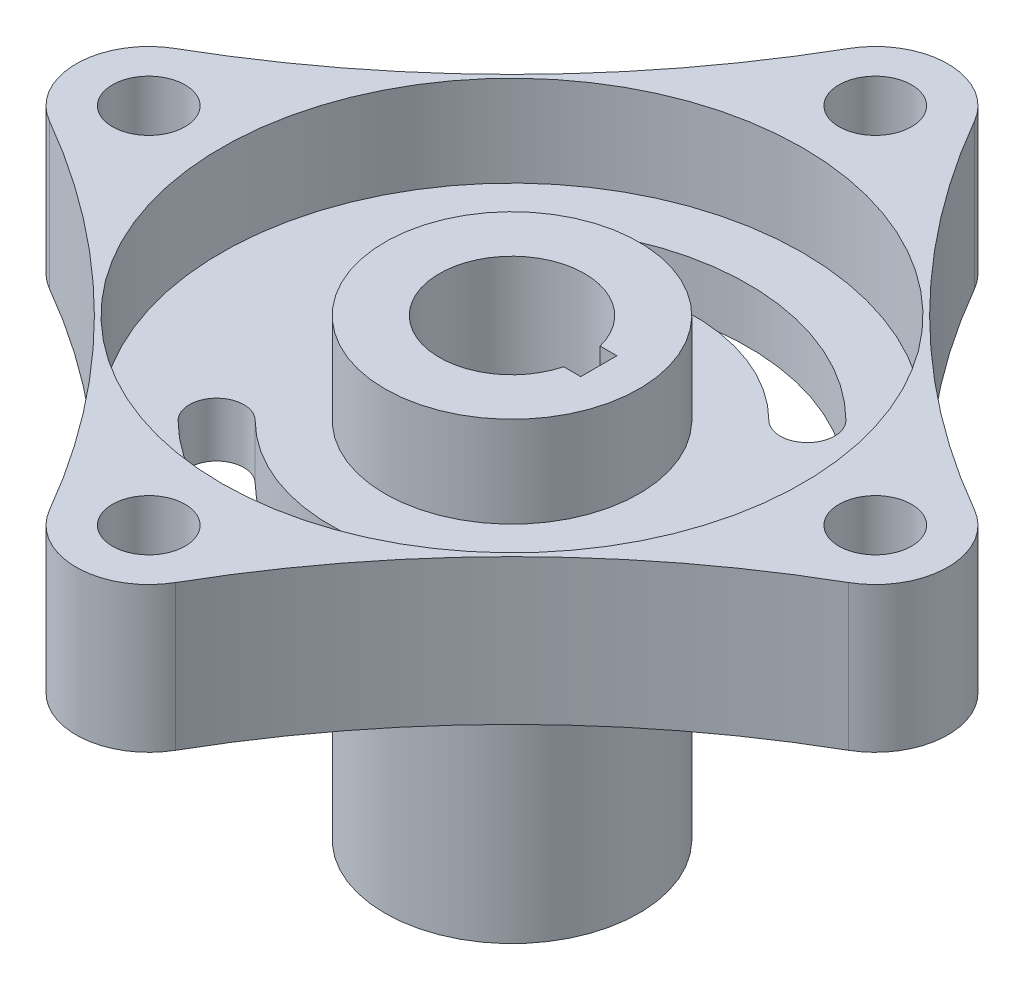
ISO-10303-21;
HEADER;
FILE_DESCRIPTION(('STEP AP214'),'2;1');
FILE_NAME('part.step','',(''),(''),'','','');
FILE_SCHEMA(('AUTOMOTIVE_DESIGN { 1 0 10303 214 1 1 1 1 }'));
ENDSEC;
DATA;
#1=APPLICATION_CONTEXT('core data for automotive mechanical design processes');
#2=APPLICATION_PROTOCOL_DEFINITION('international standard','automotive_design',2000,#1);
#3=PRODUCT_CONTEXT('',#1,'mechanical');
#4=PRODUCT('Part','Part','',(#3));
#5=PRODUCT_RELATED_PRODUCT_CATEGORY('part','',(#4));
#6=PRODUCT_DEFINITION_FORMATION('','',#4);
#7=PRODUCT_DEFINITION_CONTEXT('part definition',#1,'design');
#8=PRODUCT_DEFINITION('design','',#6,#7);
#9=PRODUCT_DEFINITION_SHAPE('','',#8);
#10=(LENGTH_UNIT() NAMED_UNIT(*) SI_UNIT(.MILLI.,.METRE.));
#11=(NAMED_UNIT(*) PLANE_ANGLE_UNIT() SI_UNIT($,.RADIAN.));
#12=(NAMED_UNIT(*) SI_UNIT($,.STERADIAN.) SOLID_ANGLE_UNIT());
#13=UNCERTAINTY_MEASURE_WITH_UNIT(LENGTH_MEASURE(1.E-05),#10,'distance_accuracy_value','');
#14=(GEOMETRIC_REPRESENTATION_CONTEXT(3) GLOBAL_UNCERTAINTY_ASSIGNED_CONTEXT((#13)) GLOBAL_UNIT_ASSIGNED_CONTEXT((#10,
#11,#12)) REPRESENTATION_CONTEXT('',''));
#15=CARTESIAN_POINT('',(0.,0.,0.));
#16=DIRECTION('',(0.,0.,1.));
#17=DIRECTION('',(1.,0.,0.));
#18=AXIS2_PLACEMENT_3D('',#15,#16,#17);
#19=CARTESIAN_POINT('',(66.8510515453765,0.,-46.8510515453766));
#20=DIRECTION('',(0.,1.,0.));
#21=DIRECTION('',(0.,0.,1.));
#22=AXIS2_PLACEMENT_3D('',#19,#20,#21);
#23=PLANE('',#22);
#24=CARTESIAN_POINT('',(0.,0.,0.));
#25=DIRECTION('',(0.,1.,0.));
#26=DIRECTION('',(0.,0.,1.));
#27=AXIS2_PLACEMENT_3D('',#24,#25,#26);
#28=CIRCLE('',#27,17.);
#29=CARTESIAN_POINT('',(0.,0.,17.));
#30=VERTEX_POINT('',#29);
#31=EDGE_CURVE('E52',#30,#30,#28,.T.);
#32=ORIENTED_EDGE('',*,*,#31,.T.);
#33=EDGE_LOOP('',(#32));
#34=FACE_BOUND('',#33,.T.);
#35=CARTESIAN_POINT('',(93.7021030907531,0.,-93.7021030907531));
#36=DIRECTION('',(0.,-1.,0.));
#37=DIRECTION('',(0.,0.,1.));
#38=AXIS2_PLACEMENT_3D('',#35,#36,#37);
#39=CIRCLE('',#38,100.);
#40=CARTESIAN_POINT('',(43.977933562278,0.,-6.94089652524096));
#41=VERTEX_POINT('',#40);
#42=CARTESIAN_POINT('',(6.94089652524096,0.,-43.977933562278));
#43=VERTEX_POINT('',#42);
#44=EDGE_CURVE('E316',#41,#43,#39,.T.);
#45=ORIENTED_EDGE('',*,*,#44,.F.);
#46=CARTESIAN_POINT('',(40.,0.,0.));
#47=DIRECTION('',(0.,1.,0.));
#48=DIRECTION('',(0.,0.,1.));
#49=AXIS2_PLACEMENT_3D('',#46,#47,#48);
#50=CIRCLE('',#49,7.99999999999999);
#51=CARTESIAN_POINT('',(43.9779335622779,0.,6.94089652524099));
#52=VERTEX_POINT('',#51);
#53=EDGE_CURVE('E323',#52,#41,#50,.T.);
#54=ORIENTED_EDGE('',*,*,#53,.F.);
#55=CARTESIAN_POINT('',(93.7021030907531,0.,93.7021030907531));
#56=DIRECTION('',(0.,-1.,0.));
#57=DIRECTION('',(0.,0.,-1.));
#58=AXIS2_PLACEMENT_3D('',#55,#56,#57);
#59=CIRCLE('',#58,100.);
#60=CARTESIAN_POINT('',(6.94089652524096,0.,43.977933562278));
#61=VERTEX_POINT('',#60);
#62=EDGE_CURVE('E348',#61,#52,#59,.T.);
#63=ORIENTED_EDGE('',*,*,#62,.F.);
#64=CARTESIAN_POINT('',(0.,0.,40.));
#65=DIRECTION('',(0.,1.,0.));
#66=DIRECTION('',(0.,0.,-1.));
#67=AXIS2_PLACEMENT_3D('',#64,#65,#66);
#68=CIRCLE('',#67,7.99999999999999);
#69=CARTESIAN_POINT('',(-6.94089652524095,0.,43.977933562278));
#70=VERTEX_POINT('',#69);
#71=EDGE_CURVE('E346',#70,#61,#68,.T.);
#72=ORIENTED_EDGE('',*,*,#71,.F.);
#73=CARTESIAN_POINT('',(-93.7021030907531,0.,93.7021030907531));
#74=DIRECTION('',(0.,-1.,0.));
#75=DIRECTION('',(0.,0.,1.));
#76=AXIS2_PLACEMENT_3D('',#73,#74,#75);
#77=CIRCLE('',#76,100.);
#78=CARTESIAN_POINT('',(-43.977933562278,0.,6.94089652524096));
#79=VERTEX_POINT('',#78);
#80=EDGE_CURVE('E347',#79,#70,#77,.T.);
#81=ORIENTED_EDGE('',*,*,#80,.F.);
#82=CARTESIAN_POINT('',(-40.,0.,0.));
#83=DIRECTION('',(0.,1.,0.));
#84=DIRECTION('',(0.,0.,-1.));
#85=AXIS2_PLACEMENT_3D('',#82,#83,#84);
#86=CIRCLE('',#85,7.99999999999999);
#87=CARTESIAN_POINT('',(-43.977933562278,0.,-6.94089652524096));
#88=VERTEX_POINT('',#87);
#89=EDGE_CURVE('E345',#88,#79,#86,.T.);
#90=ORIENTED_EDGE('',*,*,#89,.F.);
#91=CARTESIAN_POINT('',(-93.7021030907531,0.,-93.7021030907531));
#92=DIRECTION('',(0.,-1.,0.));
#93=DIRECTION('',(0.,0.,-1.));
#94=AXIS2_PLACEMENT_3D('',#91,#92,#93);
#95=CIRCLE('',#94,100.);
#96=CARTESIAN_POINT('',(-6.94089652524096,0.,-43.977933562278));
#97=VERTEX_POINT('',#96);
#98=EDGE_CURVE('E344',#97,#88,#95,.T.);
#99=ORIENTED_EDGE('',*,*,#98,.F.);
#100=CARTESIAN_POINT('',(0.,0.,-40.));
#101=DIRECTION('',(0.,1.,0.));
#102=DIRECTION('',(0.,0.,1.));
#103=AXIS2_PLACEMENT_3D('',#100,#101,#102);
#104=CIRCLE('',#103,7.99999999999999);
#105=EDGE_CURVE('E338',#43,#97,#104,.T.);
#106=ORIENTED_EDGE('',*,*,#105,.F.);
#107=EDGE_LOOP('',(#45,#54,#63,#72,#81,#90,#99,#106));
#108=FACE_BOUND('',#107,.T.);
#109=CARTESIAN_POINT('',(40.,0.,0.));
#110=DIRECTION('',(0.,1.,0.));
#111=DIRECTION('',(0.,0.,1.));
#112=AXIS2_PLACEMENT_3D('',#109,#110,#111);
#113=CIRCLE('',#112,4.00000000000001);
#114=CARTESIAN_POINT('',(40.,0.,4.00000000000001));
#115=VERTEX_POINT('',#114);
#116=EDGE_CURVE('E309',#115,#115,#113,.T.);
#117=ORIENTED_EDGE('',*,*,#116,.T.);
#118=EDGE_LOOP('',(#117));
#119=FACE_BOUND('',#118,.T.);
#120=CARTESIAN_POINT('',(-1.39659253553725E-13,0.,40.));
#121=DIRECTION('',(0.,1.,0.));
#122=DIRECTION('',(0.,0.,1.));
#123=AXIS2_PLACEMENT_3D('',#120,#121,#122);
#124=CIRCLE('',#123,4.00000000000001);
#125=CARTESIAN_POINT('',(-1.39659253553725E-13,0.,44.));
#126=VERTEX_POINT('',#125);
#127=EDGE_CURVE('E305',#126,#126,#124,.T.);
#128=ORIENTED_EDGE('',*,*,#127,.T.);
#129=EDGE_LOOP('',(#128));
#130=FACE_BOUND('',#129,.T.);
#131=CARTESIAN_POINT('',(-40.,0.,-2.79318507107451E-13));
#132=DIRECTION('',(0.,1.,0.));
#133=DIRECTION('',(0.,0.,1.));
#134=AXIS2_PLACEMENT_3D('',#131,#132,#133);
#135=CIRCLE('',#134,4.00000000000001);
#136=CARTESIAN_POINT('',(-40.,0.,3.99999999999973));
#137=VERTEX_POINT('',#136);
#138=EDGE_CURVE('E300',#137,#137,#135,.T.);
#139=ORIENTED_EDGE('',*,*,#138,.T.);
#140=EDGE_LOOP('',(#139));
#141=FACE_BOUND('',#140,.T.);
#142=CARTESIAN_POINT('',(4.18977760661176E-13,0.,-40.));
#143=DIRECTION('',(0.,1.,0.));
#144=DIRECTION('',(0.,0.,1.));
#145=AXIS2_PLACEMENT_3D('',#142,#143,#144);
#146=CIRCLE('',#145,4.00000000000001);
#147=CARTESIAN_POINT('',(4.18977760661176E-13,0.,-36.));
#148=VERTEX_POINT('',#147);
#149=EDGE_CURVE('E295',#148,#148,#146,.T.);
#150=ORIENTED_EDGE('',*,*,#149,.T.);
#151=EDGE_LOOP('',(#150));
#152=FACE_BOUND('',#151,.T.);
#153=CARTESIAN_POINT('',(0.,0.,0.));
#154=DIRECTION('',(0.,1.,0.));
#155=DIRECTION('',(0.,0.,1.));
#156=AXIS2_PLACEMENT_3D('',#153,#154,#155);
#157=CIRCLE('',#156,26.);
#158=CARTESIAN_POINT('',(18.3847763108502,0.,18.3847763108503));
#159=VERTEX_POINT('',#158);
#160=CARTESIAN_POINT('',(-18.3847763108502,0.,18.3847763108503));
#161=VERTEX_POINT('',#160);
#162=EDGE_CURVE('E225',#159,#161,#157,.F.);
#163=ORIENTED_EDGE('',*,*,#162,.F.);
#164=CARTESIAN_POINT('',(16.2634559672906,0.,16.2634559672906));
#165=DIRECTION('',(0.,1.,0.));
#166=DIRECTION('',(0.,0.,1.));
#167=AXIS2_PLACEMENT_3D('',#164,#165,#166);
#168=CIRCLE('',#167,3.);
#169=CARTESIAN_POINT('',(14.1421356237309,0.,14.142135623731));
#170=VERTEX_POINT('',#169);
#171=EDGE_CURVE('E223',#170,#159,#168,.F.);
#172=ORIENTED_EDGE('',*,*,#171,.F.);
#173=CARTESIAN_POINT('',(0.,0.,0.));
#174=DIRECTION('',(0.,1.,0.));
#175=DIRECTION('',(0.,0.,1.));
#176=AXIS2_PLACEMENT_3D('',#173,#174,#175);
#177=CIRCLE('',#176,20.);
#178=CARTESIAN_POINT('',(-14.1421356237309,0.,14.142135623731));
#179=VERTEX_POINT('',#178);
#180=EDGE_CURVE('E244',#179,#170,#177,.T.);
#181=ORIENTED_EDGE('',*,*,#180,.F.);
#182=CARTESIAN_POINT('',(-16.2634559672906,0.,16.2634559672906));
#183=DIRECTION('',(0.,1.,0.));
#184=DIRECTION('',(0.,0.,1.));
#185=AXIS2_PLACEMENT_3D('',#182,#183,#184);
#186=CIRCLE('',#185,3.);
#187=EDGE_CURVE('E67',#161,#179,#186,.F.);
#188=ORIENTED_EDGE('',*,*,#187,.F.);
#189=EDGE_LOOP('',(#163,#172,#181,#188));
#190=FACE_BOUND('',#189,.T.);
#191=CARTESIAN_POINT('',(0.,0.,0.));
#192=DIRECTION('',(0.,1.,0.));
#193=DIRECTION('',(0.,0.,1.));
#194=AXIS2_PLACEMENT_3D('',#191,#192,#193);
#195=CIRCLE('',#194,20.);
#196=CARTESIAN_POINT('',(14.1421356237309,0.,-14.142135623731));
#197=VERTEX_POINT('',#196);
#198=CARTESIAN_POINT('',(-14.1421356237309,0.,-14.142135623731));
#199=VERTEX_POINT('',#198);
#200=EDGE_CURVE('E204',#197,#199,#195,.T.);
#201=ORIENTED_EDGE('',*,*,#200,.F.);
#202=CARTESIAN_POINT('',(16.2634559672906,0.,-16.2634559672906));
#203=DIRECTION('',(0.,1.,0.));
#204=DIRECTION('',(0.,0.,1.));
#205=AXIS2_PLACEMENT_3D('',#202,#203,#204);
#206=CIRCLE('',#205,3.);
#207=CARTESIAN_POINT('',(18.3847763108502,0.,-18.3847763108503));
#208=VERTEX_POINT('',#207);
#209=EDGE_CURVE('E187',#208,#197,#206,.F.);
#210=ORIENTED_EDGE('',*,*,#209,.F.);
#211=CARTESIAN_POINT('',(0.,0.,0.));
#212=DIRECTION('',(0.,1.,0.));
#213=DIRECTION('',(0.,0.,1.));
#214=AXIS2_PLACEMENT_3D('',#211,#212,#213);
#215=CIRCLE('',#214,26.);
#216=CARTESIAN_POINT('',(-18.3847763108502,0.,-18.3847763108503));
#217=VERTEX_POINT('',#216);
#218=EDGE_CURVE('E197',#217,#208,#215,.F.);
#219=ORIENTED_EDGE('',*,*,#218,.F.);
#220=CARTESIAN_POINT('',(-16.2634559672906,0.,-16.2634559672906));
#221=DIRECTION('',(0.,1.,0.));
#222=DIRECTION('',(0.,0.,1.));
#223=AXIS2_PLACEMENT_3D('',#220,#221,#222);
#224=CIRCLE('',#223,3.);
#225=EDGE_CURVE('E58',#199,#217,#224,.F.);
#226=ORIENTED_EDGE('',*,*,#225,.F.);
#227=EDGE_LOOP('',(#201,#210,#219,#226));
#228=FACE_BOUND('',#227,.T.);
#229=ADVANCED_FACE('F44',(#34,#108,#119,#130,#141,#152,#190,#228),#23,.F.);
#230=CARTESIAN_POINT('',(0.,6.,0.));
#231=DIRECTION('',(0.,1.,0.));
#232=DIRECTION('',(0.,0.,1.));
#233=AXIS2_PLACEMENT_3D('',#230,#231,#232);
#234=PLANE('',#233);
#235=CARTESIAN_POINT('',(16.2634559672906,6.,16.2634559672906));
#236=DIRECTION('',(0.,1.,0.));
#237=DIRECTION('',(0.,0.,-1.));
#238=AXIS2_PLACEMENT_3D('',#235,#236,#237);
#239=CIRCLE('',#238,3.);
#240=CARTESIAN_POINT('',(18.3847763108502,6.,18.3847763108503));
#241=VERTEX_POINT('',#240);
#242=CARTESIAN_POINT('',(14.1421356237309,6.,14.142135623731));
#243=VERTEX_POINT('',#242);
#244=EDGE_CURVE('E230',#241,#243,#239,.T.);
#245=ORIENTED_EDGE('',*,*,#244,.F.);
#246=CARTESIAN_POINT('',(0.,6.,0.));
#247=DIRECTION('',(0.,1.,0.));
#248=DIRECTION('',(0.,0.,-1.));
#249=AXIS2_PLACEMENT_3D('',#246,#247,#248);
#250=CIRCLE('',#249,26.);
#251=CARTESIAN_POINT('',(-18.3847763108502,6.,18.3847763108503));
#252=VERTEX_POINT('',#251);
#253=EDGE_CURVE('E237',#252,#241,#250,.T.);
#254=ORIENTED_EDGE('',*,*,#253,.F.);
#255=CARTESIAN_POINT('',(-16.2634559672906,6.,16.2634559672906));
#256=DIRECTION('',(0.,1.,0.));
#257=DIRECTION('',(0.,0.,-1.));
#258=AXIS2_PLACEMENT_3D('',#255,#256,#257);
#259=CIRCLE('',#258,3.);
#260=CARTESIAN_POINT('',(-14.1421356237309,6.,14.142135623731));
#261=VERTEX_POINT('',#260);
#262=EDGE_CURVE('E232',#261,#252,#259,.T.);
#263=ORIENTED_EDGE('',*,*,#262,.F.);
#264=CARTESIAN_POINT('',(0.,6.,0.));
#265=DIRECTION('',(0.,-1.,0.));
#266=DIRECTION('',(0.,0.,-1.));
#267=AXIS2_PLACEMENT_3D('',#264,#265,#266);
#268=CIRCLE('',#267,20.);
#269=EDGE_CURVE('E228',#243,#261,#268,.T.);
#270=ORIENTED_EDGE('',*,*,#269,.F.);
#271=EDGE_LOOP('',(#245,#254,#263,#270));
#272=FACE_BOUND('',#271,.T.);
#273=CARTESIAN_POINT('',(0.,6.,0.));
#274=DIRECTION('',(0.,1.,0.));
#275=DIRECTION('',(0.,0.,1.));
#276=AXIS2_PLACEMENT_3D('',#273,#274,#275);
#277=CIRCLE('',#276,14.);
#278=CARTESIAN_POINT('',(0.,6.,14.));
#279=VERTEX_POINT('',#278);
#280=EDGE_CURVE('E376',#279,#279,#277,.T.);
#281=ORIENTED_EDGE('',*,*,#280,.F.);
#282=EDGE_LOOP('',(#281));
#283=FACE_BOUND('',#282,.T.);
#284=CARTESIAN_POINT('',(0.,6.,0.));
#285=DIRECTION('',(0.,1.,0.));
#286=DIRECTION('',(0.,0.,1.));
#287=AXIS2_PLACEMENT_3D('',#284,#285,#286);
#288=CIRCLE('',#287,32.);
#289=CARTESIAN_POINT('',(0.,6.,32.));
#290=VERTEX_POINT('',#289);
#291=EDGE_CURVE('E290',#290,#290,#288,.T.);
#292=ORIENTED_EDGE('',*,*,#291,.T.);
#293=EDGE_LOOP('',(#292));
#294=FACE_BOUND('',#293,.T.);
#295=CARTESIAN_POINT('',(16.2634559672906,6.,-16.2634559672906));
#296=DIRECTION('',(0.,1.,0.));
#297=DIRECTION('',(0.,0.,1.));
#298=AXIS2_PLACEMENT_3D('',#295,#296,#297);
#299=CIRCLE('',#298,3.);
#300=CARTESIAN_POINT('',(14.1421356237309,6.,-14.142135623731));
#301=VERTEX_POINT('',#300);
#302=CARTESIAN_POINT('',(18.3847763108502,6.,-18.3847763108503));
#303=VERTEX_POINT('',#302);
#304=EDGE_CURVE('E186',#301,#303,#299,.T.);
#305=ORIENTED_EDGE('',*,*,#304,.F.);
#306=CARTESIAN_POINT('',(0.,6.,0.));
#307=DIRECTION('',(0.,-1.,0.));
#308=DIRECTION('',(0.,0.,1.));
#309=AXIS2_PLACEMENT_3D('',#306,#307,#308);
#310=CIRCLE('',#309,20.);
#311=CARTESIAN_POINT('',(-14.1421356237309,6.,-14.142135623731));
#312=VERTEX_POINT('',#311);
#313=EDGE_CURVE('E195',#312,#301,#310,.T.);
#314=ORIENTED_EDGE('',*,*,#313,.F.);
#315=CARTESIAN_POINT('',(-16.2634559672906,6.,-16.2634559672906));
#316=DIRECTION('',(0.,1.,0.));
#317=DIRECTION('',(0.,0.,1.));
#318=AXIS2_PLACEMENT_3D('',#315,#316,#317);
#319=CIRCLE('',#318,3.);
#320=CARTESIAN_POINT('',(-18.3847763108502,6.,-18.3847763108503));
#321=VERTEX_POINT('',#320);
#322=EDGE_CURVE('E215',#321,#312,#319,.T.);
#323=ORIENTED_EDGE('',*,*,#322,.F.);
#324=CARTESIAN_POINT('',(0.,6.,0.));
#325=DIRECTION('',(0.,1.,0.));
#326=DIRECTION('',(0.,0.,1.));
#327=AXIS2_PLACEMENT_3D('',#324,#325,#326);
#328=CIRCLE('',#327,26.);
#329=EDGE_CURVE('E206',#303,#321,#328,.T.);
#330=ORIENTED_EDGE('',*,*,#329,.F.);
#331=EDGE_LOOP('',(#305,#314,#323,#330));
#332=FACE_BOUND('',#331,.T.);
#333=ADVANCED_FACE('F402',(#272,#283,#294,#332),#234,.T.);
#334=CARTESIAN_POINT('',(66.8510515453765,16.,-46.8510515453766));
#335=DIRECTION('',(0.,1.,0.));
#336=DIRECTION('',(0.,0.,1.));
#337=AXIS2_PLACEMENT_3D('',#334,#335,#336);
#338=PLANE('',#337);
#339=CARTESIAN_POINT('',(0.,16.,0.));
#340=DIRECTION('',(0.,1.,0.));
#341=DIRECTION('',(0.,0.,1.));
#342=AXIS2_PLACEMENT_3D('',#339,#340,#341);
#343=CIRCLE('',#342,32.);
#344=CARTESIAN_POINT('',(0.,16.,32.));
#345=VERTEX_POINT('',#344);
#346=EDGE_CURVE('E287',#345,#345,#343,.T.);
#347=ORIENTED_EDGE('',*,*,#346,.F.);
#348=EDGE_LOOP('',(#347));
#349=FACE_BOUND('',#348,.T.);
#350=CARTESIAN_POINT('',(-40.,16.,-2.79318507107451E-13));
#351=DIRECTION('',(0.,1.,0.));
#352=DIRECTION('',(0.,0.,1.));
#353=AXIS2_PLACEMENT_3D('',#350,#351,#352);
#354=CIRCLE('',#353,4.00000000000001);
#355=CARTESIAN_POINT('',(-40.,16.,3.99999999999973));
#356=VERTEX_POINT('',#355);
#357=EDGE_CURVE('E303',#356,#356,#354,.T.);
#358=ORIENTED_EDGE('',*,*,#357,.F.);
#359=EDGE_LOOP('',(#358));
#360=FACE_BOUND('',#359,.T.);
#361=CARTESIAN_POINT('',(40.,16.,0.));
#362=DIRECTION('',(0.,1.,0.));
#363=DIRECTION('',(0.,0.,1.));
#364=AXIS2_PLACEMENT_3D('',#361,#362,#363);
#365=CIRCLE('',#364,4.00000000000001);
#366=CARTESIAN_POINT('',(40.,16.,4.00000000000001));
#367=VERTEX_POINT('',#366);
#368=EDGE_CURVE('E311',#367,#367,#365,.T.);
#369=ORIENTED_EDGE('',*,*,#368,.F.);
#370=EDGE_LOOP('',(#369));
#371=FACE_BOUND('',#370,.T.);
#372=CARTESIAN_POINT('',(93.7021030907531,16.,-93.7021030907531));
#373=DIRECTION('',(0.,-1.,0.));
#374=DIRECTION('',(0.,0.,1.));
#375=AXIS2_PLACEMENT_3D('',#372,#373,#374);
#376=CIRCLE('',#375,100.);
#377=CARTESIAN_POINT('',(43.977933562278,16.,-6.94089652524096));
#378=VERTEX_POINT('',#377);
#379=CARTESIAN_POINT('',(6.94089652524096,16.,-43.977933562278));
#380=VERTEX_POINT('',#379);
#381=EDGE_CURVE('E317',#378,#380,#376,.T.);
#382=ORIENTED_EDGE('',*,*,#381,.T.);
#383=CARTESIAN_POINT('',(0.,16.,-40.));
#384=DIRECTION('',(0.,1.,0.));
#385=DIRECTION('',(0.,0.,1.));
#386=AXIS2_PLACEMENT_3D('',#383,#384,#385);
#387=CIRCLE('',#386,7.99999999999999);
#388=CARTESIAN_POINT('',(-6.94089652524096,16.,-43.977933562278));
#389=VERTEX_POINT('',#388);
#390=EDGE_CURVE('E325',#380,#389,#387,.T.);
#391=ORIENTED_EDGE('',*,*,#390,.T.);
#392=CARTESIAN_POINT('',(-93.7021030907531,16.,-93.7021030907531));
#393=DIRECTION('',(0.,-1.,0.));
#394=DIRECTION('',(0.,0.,-1.));
#395=AXIS2_PLACEMENT_3D('',#392,#393,#394);
#396=CIRCLE('',#395,100.);
#397=CARTESIAN_POINT('',(-43.977933562278,16.,-6.94089652524096));
#398=VERTEX_POINT('',#397);
#399=EDGE_CURVE('E324',#389,#398,#396,.T.);
#400=ORIENTED_EDGE('',*,*,#399,.T.);
#401=CARTESIAN_POINT('',(-40.,16.,0.));
#402=DIRECTION('',(0.,1.,0.));
#403=DIRECTION('',(0.,0.,-1.));
#404=AXIS2_PLACEMENT_3D('',#401,#402,#403);
#405=CIRCLE('',#404,7.99999999999999);
#406=CARTESIAN_POINT('',(-43.977933562278,16.,6.94089652524096));
#407=VERTEX_POINT('',#406);
#408=EDGE_CURVE('E330',#398,#407,#405,.T.);
#409=ORIENTED_EDGE('',*,*,#408,.T.);
#410=CARTESIAN_POINT('',(-93.7021030907531,16.,93.7021030907531));
#411=DIRECTION('',(0.,-1.,0.));
#412=DIRECTION('',(0.,0.,1.));
#413=AXIS2_PLACEMENT_3D('',#410,#411,#412);
#414=CIRCLE('',#413,100.);
#415=CARTESIAN_POINT('',(-6.94089652524095,16.,43.977933562278));
#416=VERTEX_POINT('',#415);
#417=EDGE_CURVE('E328',#407,#416,#414,.T.);
#418=ORIENTED_EDGE('',*,*,#417,.T.);
#419=CARTESIAN_POINT('',(0.,16.,40.));
#420=DIRECTION('',(0.,1.,0.));
#421=DIRECTION('',(0.,0.,-1.));
#422=AXIS2_PLACEMENT_3D('',#419,#420,#421);
#423=CIRCLE('',#422,7.99999999999999);
#424=CARTESIAN_POINT('',(6.94089652524096,16.,43.977933562278));
#425=VERTEX_POINT('',#424);
#426=EDGE_CURVE('E332',#416,#425,#423,.T.);
#427=ORIENTED_EDGE('',*,*,#426,.T.);
#428=CARTESIAN_POINT('',(93.7021030907531,16.,93.7021030907531));
#429=DIRECTION('',(0.,-1.,0.));
#430=DIRECTION('',(0.,0.,-1.));
#431=AXIS2_PLACEMENT_3D('',#428,#429,#430);
#432=CIRCLE('',#431,100.);
#433=CARTESIAN_POINT('',(43.9779335622779,16.,6.94089652524099));
#434=VERTEX_POINT('',#433);
#435=EDGE_CURVE('E334',#425,#434,#432,.T.);
#436=ORIENTED_EDGE('',*,*,#435,.T.);
#437=CARTESIAN_POINT('',(40.,16.,0.));
#438=DIRECTION('',(0.,1.,0.));
#439=DIRECTION('',(0.,0.,1.));
#440=AXIS2_PLACEMENT_3D('',#437,#438,#439);
#441=CIRCLE('',#440,7.99999999999999);
#442=EDGE_CURVE('E333',#434,#378,#441,.T.);
#443=ORIENTED_EDGE('',*,*,#442,.T.);
#444=EDGE_LOOP('',(#382,#391,#400,#409,#418,#427,#436,#443));
#445=FACE_BOUND('',#444,.T.);
#446=CARTESIAN_POINT('',(-1.39659253553725E-13,16.,40.));
#447=DIRECTION('',(0.,1.,0.));
#448=DIRECTION('',(0.,0.,1.));
#449=AXIS2_PLACEMENT_3D('',#446,#447,#448);
#450=CIRCLE('',#449,4.00000000000001);
#451=CARTESIAN_POINT('',(-1.39659253553725E-13,16.,44.));
#452=VERTEX_POINT('',#451);
#453=EDGE_CURVE('E307',#452,#452,#450,.T.);
#454=ORIENTED_EDGE('',*,*,#453,.F.);
#455=EDGE_LOOP('',(#454));
#456=FACE_BOUND('',#455,.T.);
#457=CARTESIAN_POINT('',(4.18977760661176E-13,16.,-40.));
#458=DIRECTION('',(0.,1.,0.));
#459=DIRECTION('',(0.,0.,1.));
#460=AXIS2_PLACEMENT_3D('',#457,#458,#459);
#461=CIRCLE('',#460,4.00000000000001);
#462=CARTESIAN_POINT('',(4.18977760661176E-13,16.,-36.));
#463=VERTEX_POINT('',#462);
#464=EDGE_CURVE('E293',#463,#463,#461,.T.);
#465=ORIENTED_EDGE('',*,*,#464,.F.);
#466=EDGE_LOOP('',(#465));
#467=FACE_BOUND('',#466,.T.);
#468=ADVANCED_FACE('F409',(#349,#360,#371,#445,#456,#467),#338,.T.);
#469=CARTESIAN_POINT('',(93.7021030907531,16.,-93.7021030907531));
#470=DIRECTION('',(0.,-1.,0.));
#471=DIRECTION('',(0.,0.,-1.));
#472=AXIS2_PLACEMENT_3D('',#469,#470,#471);
#473=CYLINDRICAL_SURFACE('',#472,100.);
#474=ORIENTED_EDGE('',*,*,#44,.T.);
#475=DIRECTION('',(0.,-1.,0.));
#476=VECTOR('',#475,1.);
#477=CARTESIAN_POINT('',(6.94089652524096,16.,-43.977933562278));
#478=LINE('',#477,#476);
#479=EDGE_CURVE('E373',#380,#43,#478,.T.);
#480=ORIENTED_EDGE('',*,*,#479,.F.);
#481=ORIENTED_EDGE('',*,*,#381,.F.);
#482=DIRECTION('',(0.,-1.,0.));
#483=VECTOR('',#482,1.);
#484=CARTESIAN_POINT('',(43.977933562278,16.,-6.94089652524096));
#485=LINE('',#484,#483);
#486=EDGE_CURVE('E339',#378,#41,#485,.T.);
#487=ORIENTED_EDGE('',*,*,#486,.T.);
#488=EDGE_LOOP('',(#474,#480,#481,#487));
#489=FACE_BOUND('',#488,.T.);
#490=ADVANCED_FACE('F439',(#489),#473,.F.);
#491=CARTESIAN_POINT('',(0.,16.,-40.));
#492=DIRECTION('',(0.,-1.,0.));
#493=DIRECTION('',(0.,0.,-1.));
#494=AXIS2_PLACEMENT_3D('',#491,#492,#493);
#495=CYLINDRICAL_SURFACE('',#494,7.99999999999999);
#496=ORIENTED_EDGE('',*,*,#105,.T.);
#497=DIRECTION('',(0.,-1.,0.));
#498=VECTOR('',#497,1.);
#499=CARTESIAN_POINT('',(-6.94089652524096,16.,-43.977933562278));
#500=LINE('',#499,#498);
#501=EDGE_CURVE('E367',#389,#97,#500,.T.);
#502=ORIENTED_EDGE('',*,*,#501,.F.);
#503=ORIENTED_EDGE('',*,*,#390,.F.);
#504=ORIENTED_EDGE('',*,*,#479,.T.);
#505=EDGE_LOOP('',(#496,#502,#503,#504));
#506=FACE_BOUND('',#505,.T.);
#507=ADVANCED_FACE('F440',(#506),#495,.T.);
#508=CARTESIAN_POINT('',(-93.7021030907531,16.,-93.7021030907531));
#509=DIRECTION('',(0.,-1.,0.));
#510=DIRECTION('',(0.,0.,-1.));
#511=AXIS2_PLACEMENT_3D('',#508,#509,#510);
#512=CYLINDRICAL_SURFACE('',#511,100.);
#513=ORIENTED_EDGE('',*,*,#98,.T.);
#514=DIRECTION('',(0.,-1.,0.));
#515=VECTOR('',#514,1.);
#516=CARTESIAN_POINT('',(-43.977933562278,16.,-6.94089652524096));
#517=LINE('',#516,#515);
#518=EDGE_CURVE('E370',#398,#88,#517,.T.);
#519=ORIENTED_EDGE('',*,*,#518,.F.);
#520=ORIENTED_EDGE('',*,*,#399,.F.);
#521=ORIENTED_EDGE('',*,*,#501,.T.);
#522=EDGE_LOOP('',(#513,#519,#520,#521));
#523=FACE_BOUND('',#522,.T.);
#524=ADVANCED_FACE('F433',(#523),#512,.F.);
#525=CARTESIAN_POINT('',(-40.,16.,0.));
#526=DIRECTION('',(0.,-1.,0.));
#527=DIRECTION('',(0.,0.,-1.));
#528=AXIS2_PLACEMENT_3D('',#525,#526,#527);
#529=CYLINDRICAL_SURFACE('',#528,7.99999999999999);
#530=ORIENTED_EDGE('',*,*,#89,.T.);
#531=DIRECTION('',(0.,-1.,0.));
#532=VECTOR('',#531,1.);
#533=CARTESIAN_POINT('',(-43.977933562278,16.,6.94089652524096));
#534=LINE('',#533,#532);
#535=EDGE_CURVE('E365',#407,#79,#534,.T.);
#536=ORIENTED_EDGE('',*,*,#535,.F.);
#537=ORIENTED_EDGE('',*,*,#408,.F.);
#538=ORIENTED_EDGE('',*,*,#518,.T.);
#539=EDGE_LOOP('',(#530,#536,#537,#538));
#540=FACE_BOUND('',#539,.T.);
#541=ADVANCED_FACE('F427',(#540),#529,.T.);
#542=CARTESIAN_POINT('',(-93.7021030907531,16.,93.7021030907531));
#543=DIRECTION('',(0.,-1.,0.));
#544=DIRECTION('',(0.,0.,-1.));
#545=AXIS2_PLACEMENT_3D('',#542,#543,#544);
#546=CYLINDRICAL_SURFACE('',#545,100.);
#547=ORIENTED_EDGE('',*,*,#80,.T.);
#548=DIRECTION('',(0.,-1.,0.));
#549=VECTOR('',#548,1.);
#550=CARTESIAN_POINT('',(-6.94089652524095,16.,43.977933562278));
#551=LINE('',#550,#549);
#552=EDGE_CURVE('E363',#416,#70,#551,.T.);
#553=ORIENTED_EDGE('',*,*,#552,.F.);
#554=ORIENTED_EDGE('',*,*,#417,.F.);
#555=ORIENTED_EDGE('',*,*,#535,.T.);
#556=EDGE_LOOP('',(#547,#553,#554,#555));
#557=FACE_BOUND('',#556,.T.);
#558=ADVANCED_FACE('F422',(#557),#546,.F.);
#559=CARTESIAN_POINT('',(0.,16.,40.));
#560=DIRECTION('',(0.,-1.,0.));
#561=DIRECTION('',(0.,0.,-1.));
#562=AXIS2_PLACEMENT_3D('',#559,#560,#561);
#563=CYLINDRICAL_SURFACE('',#562,7.99999999999999);
#564=ORIENTED_EDGE('',*,*,#71,.T.);
#565=DIRECTION('',(0.,-1.,0.));
#566=VECTOR('',#565,1.);
#567=CARTESIAN_POINT('',(6.94089652524096,16.,43.977933562278));
#568=LINE('',#567,#566);
#569=EDGE_CURVE('E357',#425,#61,#568,.T.);
#570=ORIENTED_EDGE('',*,*,#569,.F.);
#571=ORIENTED_EDGE('',*,*,#426,.F.);
#572=ORIENTED_EDGE('',*,*,#552,.T.);
#573=EDGE_LOOP('',(#564,#570,#571,#572));
#574=FACE_BOUND('',#573,.T.);
#575=ADVANCED_FACE('F423',(#574),#563,.T.);
#576=CARTESIAN_POINT('',(93.7021030907531,16.,93.7021030907531));
#577=DIRECTION('',(0.,-1.,0.));
#578=DIRECTION('',(0.,0.,-1.));
#579=AXIS2_PLACEMENT_3D('',#576,#577,#578);
#580=CYLINDRICAL_SURFACE('',#579,100.);
#581=ORIENTED_EDGE('',*,*,#62,.T.);
#582=DIRECTION('',(0.,-1.,0.));
#583=VECTOR('',#582,1.);
#584=CARTESIAN_POINT('',(43.9779335622779,16.,6.94089652524099));
#585=LINE('',#584,#583);
#586=EDGE_CURVE('E353',#434,#52,#585,.T.);
#587=ORIENTED_EDGE('',*,*,#586,.F.);
#588=ORIENTED_EDGE('',*,*,#435,.F.);
#589=ORIENTED_EDGE('',*,*,#569,.T.);
#590=EDGE_LOOP('',(#581,#587,#588,#589));
#591=FACE_BOUND('',#590,.T.);
#592=ADVANCED_FACE('F417',(#591),#580,.F.);
#593=CARTESIAN_POINT('',(40.,16.,0.));
#594=DIRECTION('',(0.,-1.,0.));
#595=DIRECTION('',(0.,0.,-1.));
#596=AXIS2_PLACEMENT_3D('',#593,#594,#595);
#597=CYLINDRICAL_SURFACE('',#596,7.99999999999999);
#598=ORIENTED_EDGE('',*,*,#53,.T.);
#599=ORIENTED_EDGE('',*,*,#486,.F.);
#600=ORIENTED_EDGE('',*,*,#442,.F.);
#601=ORIENTED_EDGE('',*,*,#586,.T.);
#602=EDGE_LOOP('',(#598,#599,#600,#601));
#603=FACE_BOUND('',#602,.T.);
#604=ADVANCED_FACE('F412',(#603),#597,.T.);
#605=CARTESIAN_POINT('',(40.,16.,0.));
#606=DIRECTION('',(0.,-1.,0.));
#607=DIRECTION('',(0.,0.,-1.));
#608=AXIS2_PLACEMENT_3D('',#605,#606,#607);
#609=CYLINDRICAL_SURFACE('',#608,4.00000000000001);
#610=ORIENTED_EDGE('',*,*,#368,.T.);
#611=EDGE_LOOP('',(#610));
#612=FACE_BOUND('',#611,.T.);
#613=ORIENTED_EDGE('',*,*,#116,.F.);
#614=EDGE_LOOP('',(#613));
#615=FACE_BOUND('',#614,.T.);
#616=ADVANCED_FACE('F418',(#612,#615),#609,.F.);
#617=CARTESIAN_POINT('',(-1.39659253553725E-13,16.,40.));
#618=DIRECTION('',(0.,-1.,0.));
#619=DIRECTION('',(0.,0.,-1.));
#620=AXIS2_PLACEMENT_3D('',#617,#618,#619);
#621=CYLINDRICAL_SURFACE('',#620,4.00000000000001);
#622=ORIENTED_EDGE('',*,*,#453,.T.);
#623=EDGE_LOOP('',(#622));
#624=FACE_BOUND('',#623,.T.);
#625=ORIENTED_EDGE('',*,*,#127,.F.);
#626=EDGE_LOOP('',(#625));
#627=FACE_BOUND('',#626,.T.);
#628=ADVANCED_FACE('F555',(#624,#627),#621,.F.);
#629=CARTESIAN_POINT('',(-40.,16.,-2.79318507107451E-13));
#630=DIRECTION('',(0.,-1.,0.));
#631=DIRECTION('',(0.,0.,-1.));
#632=AXIS2_PLACEMENT_3D('',#629,#630,#631);
#633=CYLINDRICAL_SURFACE('',#632,4.00000000000001);
#634=ORIENTED_EDGE('',*,*,#357,.T.);
#635=EDGE_LOOP('',(#634));
#636=FACE_BOUND('',#635,.T.);
#637=ORIENTED_EDGE('',*,*,#138,.F.);
#638=EDGE_LOOP('',(#637));
#639=FACE_BOUND('',#638,.T.);
#640=ADVANCED_FACE('F481',(#636,#639),#633,.F.);
#641=CARTESIAN_POINT('',(4.18977760661176E-13,16.,-40.));
#642=DIRECTION('',(0.,-1.,0.));
#643=DIRECTION('',(0.,0.,-1.));
#644=AXIS2_PLACEMENT_3D('',#641,#642,#643);
#645=CYLINDRICAL_SURFACE('',#644,4.00000000000001);
#646=ORIENTED_EDGE('',*,*,#464,.T.);
#647=EDGE_LOOP('',(#646));
#648=FACE_BOUND('',#647,.T.);
#649=ORIENTED_EDGE('',*,*,#149,.F.);
#650=EDGE_LOOP('',(#649));
#651=FACE_BOUND('',#650,.T.);
#652=ADVANCED_FACE('F480',(#648,#651),#645,.F.);
#653=CARTESIAN_POINT('',(0.,6.,0.));
#654=DIRECTION('',(0.,1.,0.));
#655=DIRECTION('',(0.,0.,1.));
#656=AXIS2_PLACEMENT_3D('',#653,#654,#655);
#657=CYLINDRICAL_SURFACE('',#656,32.);
#658=ORIENTED_EDGE('',*,*,#291,.F.);
#659=EDGE_LOOP('',(#658));
#660=FACE_BOUND('',#659,.T.);
#661=ORIENTED_EDGE('',*,*,#346,.T.);
#662=EDGE_LOOP('',(#661));
#663=FACE_BOUND('',#662,.T.);
#664=ADVANCED_FACE('F477',(#660,#663),#657,.F.);
#665=CARTESIAN_POINT('',(66.8510515453765,16.,-46.8510515453766));
#666=DIRECTION('',(0.,1.,0.));
#667=DIRECTION('',(0.,0.,1.));
#668=AXIS2_PLACEMENT_3D('',#665,#666,#667);
#669=PLANE('',#668);
#670=CARTESIAN_POINT('',(0.,16.,0.));
#671=DIRECTION('',(0.,1.,0.));
#672=DIRECTION('',(0.,0.,1.));
#673=AXIS2_PLACEMENT_3D('',#670,#671,#672);
#674=CIRCLE('',#673,8.);
#675=CARTESIAN_POINT('',(7.76183003524167,16.,-1.93752277509718));
#676=VERTEX_POINT('',#675);
#677=CARTESIAN_POINT('',(7.73487471041085,16.,2.04247722490282));
#678=VERTEX_POINT('',#677);
#679=EDGE_CURVE('E199',#676,#678,#674,.T.);
#680=ORIENTED_EDGE('',*,*,#679,.F.);
#681=DIRECTION('',(-1.,0.,0.));
#682=VECTOR('',#681,1.);
#683=CARTESIAN_POINT('',(9.61183003524167,16.,-1.93752277509718));
#684=LINE('',#683,#682);
#685=CARTESIAN_POINT('',(9.61183003524167,16.,-1.93752277509718));
#686=VERTEX_POINT('',#685);
#687=EDGE_CURVE('E254',#686,#676,#684,.T.);
#688=ORIENTED_EDGE('',*,*,#687,.F.);
#689=DIRECTION('',(0.,0.,-1.));
#690=VECTOR('',#689,1.);
#691=CARTESIAN_POINT('',(9.61183003524167,16.,0.));
#692=LINE('',#691,#690);
#693=CARTESIAN_POINT('',(9.61183003524167,16.,2.04247722490282));
#694=VERTEX_POINT('',#693);
#695=EDGE_CURVE('E267',#694,#686,#692,.T.);
#696=ORIENTED_EDGE('',*,*,#695,.F.);
#697=DIRECTION('',(1.,0.,0.));
#698=VECTOR('',#697,1.);
#699=CARTESIAN_POINT('',(9.61183003524167,16.,2.04247722490282));
#700=LINE('',#699,#698);
#701=EDGE_CURVE('E266',#678,#694,#700,.T.);
#702=ORIENTED_EDGE('',*,*,#701,.F.);
#703=EDGE_LOOP('',(#680,#688,#696,#702));
#704=FACE_BOUND('',#703,.T.);
#705=CARTESIAN_POINT('',(0.,16.,0.));
#706=DIRECTION('',(0.,1.,0.));
#707=DIRECTION('',(0.,0.,1.));
#708=AXIS2_PLACEMENT_3D('',#705,#706,#707);
#709=CIRCLE('',#708,14.);
#710=CARTESIAN_POINT('',(0.,16.,14.));
#711=VERTEX_POINT('',#710);
#712=EDGE_CURVE('E277',#711,#711,#709,.T.);
#713=ORIENTED_EDGE('',*,*,#712,.T.);
#714=EDGE_LOOP('',(#713));
#715=FACE_BOUND('',#714,.T.);
#716=ADVANCED_FACE('F539',(#704,#715),#669,.T.);
#717=CARTESIAN_POINT('',(0.,-34.,0.));
#718=DIRECTION('',(0.,1.,0.));
#719=DIRECTION('',(0.,0.,1.));
#720=AXIS2_PLACEMENT_3D('',#717,#718,#719);
#721=CYLINDRICAL_SURFACE('',#720,14.);
#722=ORIENTED_EDGE('',*,*,#280,.T.);
#723=EDGE_LOOP('',(#722));
#724=FACE_BOUND('',#723,.T.);
#725=ORIENTED_EDGE('',*,*,#712,.F.);
#726=EDGE_LOOP('',(#725));
#727=FACE_BOUND('',#726,.T.);
#728=ADVANCED_FACE('F541',(#724,#727),#721,.T.);
#729=CARTESIAN_POINT('',(0.,-3.,0.));
#730=DIRECTION('',(0.,1.,0.));
#731=DIRECTION('',(0.,0.,1.));
#732=AXIS2_PLACEMENT_3D('',#729,#730,#731);
#733=CIRCLE('',#732,14.);
#734=CARTESIAN_POINT('',(0.,-3.,14.));
#735=VERTEX_POINT('',#734);
#736=EDGE_CURVE('E11',#735,#735,#733,.F.);
#737=ORIENTED_EDGE('',*,*,#736,.T.);
#738=EDGE_LOOP('',(#737));
#739=FACE_BOUND('',#738,.T.);
#740=CARTESIAN_POINT('',(0.,-34.,0.));
#741=DIRECTION('',(0.,1.,0.));
#742=DIRECTION('',(0.,0.,1.));
#743=AXIS2_PLACEMENT_3D('',#740,#741,#742);
#744=CIRCLE('',#743,14.);
#745=CARTESIAN_POINT('',(0.,-34.,14.));
#746=VERTEX_POINT('',#745);
#747=EDGE_CURVE('E283',#746,#746,#744,.T.);
#748=ORIENTED_EDGE('',*,*,#747,.T.);
#749=EDGE_LOOP('',(#748));
#750=FACE_BOUND('',#749,.T.);
#751=ADVANCED_FACE('F398',(#739,#750),#721,.T.);
#752=CARTESIAN_POINT('',(0.,-34.,0.));
#753=DIRECTION('',(0.,1.,0.));
#754=DIRECTION('',(0.,0.,1.));
#755=AXIS2_PLACEMENT_3D('',#752,#753,#754);
#756=PLANE('',#755);
#757=DIRECTION('',(-1.,0.,0.));
#758=VECTOR('',#757,1.);
#759=CARTESIAN_POINT('',(9.61183003524167,-34.,-1.93752277509718));
#760=LINE('',#759,#758);
#761=CARTESIAN_POINT('',(9.61183003524167,-34.,-1.93752277509718));
#762=VERTEX_POINT('',#761);
#763=CARTESIAN_POINT('',(7.76183003524167,-34.,-1.93752277509718));
#764=VERTEX_POINT('',#763);
#765=EDGE_CURVE('E261',#762,#764,#760,.T.);
#766=ORIENTED_EDGE('',*,*,#765,.T.);
#767=CARTESIAN_POINT('',(0.,-34.,0.));
#768=DIRECTION('',(0.,1.,0.));
#769=DIRECTION('',(0.,0.,1.));
#770=AXIS2_PLACEMENT_3D('',#767,#768,#769);
#771=CIRCLE('',#770,8.);
#772=CARTESIAN_POINT('',(7.73487471041085,-34.,2.04247722490282));
#773=VERTEX_POINT('',#772);
#774=EDGE_CURVE('E253',#764,#773,#771,.T.);
#775=ORIENTED_EDGE('',*,*,#774,.T.);
#776=DIRECTION('',(1.,0.,0.));
#777=VECTOR('',#776,1.);
#778=CARTESIAN_POINT('',(9.61183003524167,-34.,2.04247722490282));
#779=LINE('',#778,#777);
#780=CARTESIAN_POINT('',(9.61183003524167,-34.,2.04247722490282));
#781=VERTEX_POINT('',#780);
#782=EDGE_CURVE('E255',#773,#781,#779,.T.);
#783=ORIENTED_EDGE('',*,*,#782,.T.);
#784=DIRECTION('',(0.,0.,-1.));
#785=VECTOR('',#784,1.);
#786=CARTESIAN_POINT('',(9.61183003524167,-34.,0.));
#787=LINE('',#786,#785);
#788=EDGE_CURVE('E256',#781,#762,#787,.T.);
#789=ORIENTED_EDGE('',*,*,#788,.T.);
#790=EDGE_LOOP('',(#766,#775,#783,#789));
#791=FACE_BOUND('',#790,.T.);
#792=ORIENTED_EDGE('',*,*,#747,.F.);
#793=EDGE_LOOP('',(#792));
#794=FACE_BOUND('',#793,.T.);
#795=ADVANCED_FACE('F384',(#791,#794),#756,.F.);
#796=CARTESIAN_POINT('',(0.,-3.,0.));
#797=DIRECTION('',(0.,1.,0.));
#798=DIRECTION('',(0.,0.,1.));
#799=AXIS2_PLACEMENT_3D('',#796,#797,#798);
#800=TOROIDAL_SURFACE('',#799,17.,3.);
#801=ORIENTED_EDGE('',*,*,#736,.F.);
#802=EDGE_LOOP('',(#801));
#803=FACE_BOUND('',#802,.T.);
#804=ORIENTED_EDGE('',*,*,#31,.F.);
#805=EDGE_LOOP('',(#804));
#806=FACE_BOUND('',#805,.T.);
#807=ADVANCED_FACE('F50',(#803,#806),#800,.F.);
#808=CARTESIAN_POINT('',(0.,-34.,0.));
#809=DIRECTION('',(0.,1.,0.));
#810=DIRECTION('',(0.,0.,1.));
#811=AXIS2_PLACEMENT_3D('',#808,#809,#810);
#812=CYLINDRICAL_SURFACE('',#811,8.);
#813=ORIENTED_EDGE('',*,*,#679,.T.);
#814=DIRECTION('',(0.,1.,0.));
#815=VECTOR('',#814,1.);
#816=CARTESIAN_POINT('',(7.73487471041085,-34.,2.04247722490282));
#817=LINE('',#816,#815);
#818=EDGE_CURVE('E262',#773,#678,#817,.T.);
#819=ORIENTED_EDGE('',*,*,#818,.F.);
#820=ORIENTED_EDGE('',*,*,#774,.F.);
#821=DIRECTION('',(0.,1.,0.));
#822=VECTOR('',#821,1.);
#823=CARTESIAN_POINT('',(7.76183003524167,-34.,-1.93752277509718));
#824=LINE('',#823,#822);
#825=EDGE_CURVE('E273',#764,#676,#824,.T.);
#826=ORIENTED_EDGE('',*,*,#825,.T.);
#827=EDGE_LOOP('',(#813,#819,#820,#826));
#828=FACE_BOUND('',#827,.T.);
#829=ADVANCED_FACE('F383',(#828),#812,.F.);
#830=CARTESIAN_POINT('',(9.61183003524167,-34.,-1.93752277509718));
#831=DIRECTION('',(0.,0.,-1.));
#832=DIRECTION('',(-1.,0.,0.));
#833=AXIS2_PLACEMENT_3D('',#830,#831,#832);
#834=PLANE('',#833);
#835=ORIENTED_EDGE('',*,*,#687,.T.);
#836=ORIENTED_EDGE('',*,*,#825,.F.);
#837=ORIENTED_EDGE('',*,*,#765,.F.);
#838=DIRECTION('',(0.,1.,0.));
#839=VECTOR('',#838,1.);
#840=CARTESIAN_POINT('',(9.61183003524167,-34.,-1.93752277509718));
#841=LINE('',#840,#839);
#842=EDGE_CURVE('E280',#762,#686,#841,.T.);
#843=ORIENTED_EDGE('',*,*,#842,.T.);
#844=EDGE_LOOP('',(#835,#836,#837,#843));
#845=FACE_BOUND('',#844,.T.);
#846=ADVANCED_FACE('F394',(#845),#834,.F.);
#847=CARTESIAN_POINT('',(9.61183003524167,-34.,0.));
#848=DIRECTION('',(1.,0.,0.));
#849=DIRECTION('',(0.,0.,-1.));
#850=AXIS2_PLACEMENT_3D('',#847,#848,#849);
#851=PLANE('',#850);
#852=ORIENTED_EDGE('',*,*,#695,.T.);
#853=ORIENTED_EDGE('',*,*,#842,.F.);
#854=ORIENTED_EDGE('',*,*,#788,.F.);
#855=DIRECTION('',(0.,1.,0.));
#856=VECTOR('',#855,1.);
#857=CARTESIAN_POINT('',(9.61183003524167,-34.,2.04247722490282));
#858=LINE('',#857,#856);
#859=EDGE_CURVE('E276',#781,#694,#858,.T.);
#860=ORIENTED_EDGE('',*,*,#859,.T.);
#861=EDGE_LOOP('',(#852,#853,#854,#860));
#862=FACE_BOUND('',#861,.T.);
#863=ADVANCED_FACE('F535',(#862),#851,.F.);
#864=CARTESIAN_POINT('',(9.61183003524167,-34.,2.04247722490282));
#865=DIRECTION('',(0.,0.,1.));
#866=DIRECTION('',(1.,0.,0.));
#867=AXIS2_PLACEMENT_3D('',#864,#865,#866);
#868=PLANE('',#867);
#869=ORIENTED_EDGE('',*,*,#701,.T.);
#870=ORIENTED_EDGE('',*,*,#859,.F.);
#871=ORIENTED_EDGE('',*,*,#782,.F.);
#872=ORIENTED_EDGE('',*,*,#818,.T.);
#873=EDGE_LOOP('',(#869,#870,#871,#872));
#874=FACE_BOUND('',#873,.T.);
#875=ADVANCED_FACE('F530',(#874),#868,.F.);
#876=CARTESIAN_POINT('',(16.2634559672906,-34.001,16.2634559672906));
#877=DIRECTION('',(0.,1.,0.));
#878=DIRECTION('',(0.,0.,1.));
#879=AXIS2_PLACEMENT_3D('',#876,#877,#878);
#880=CYLINDRICAL_SURFACE('',#879,3.);
#881=ORIENTED_EDGE('',*,*,#171,.T.);
#882=DIRECTION('',(0.,1.,0.));
#883=VECTOR('',#882,1.);
#884=CARTESIAN_POINT('',(18.3847763108502,-34.001,18.3847763108503));
#885=LINE('',#884,#883);
#886=EDGE_CURVE('E238',#159,#241,#885,.T.);
#887=ORIENTED_EDGE('',*,*,#886,.T.);
#888=ORIENTED_EDGE('',*,*,#244,.T.);
#889=DIRECTION('',(0.,1.,0.));
#890=VECTOR('',#889,1.);
#891=CARTESIAN_POINT('',(14.1421356237309,-34.001,14.142135623731));
#892=LINE('',#891,#890);
#893=EDGE_CURVE('E239',#170,#243,#892,.T.);
#894=ORIENTED_EDGE('',*,*,#893,.F.);
#895=EDGE_LOOP('',(#881,#887,#888,#894));
#896=FACE_BOUND('',#895,.T.);
#897=ADVANCED_FACE('F493',(#896),#880,.F.);
#898=CARTESIAN_POINT('',(0.,-34.001,0.));
#899=DIRECTION('',(0.,1.,0.));
#900=DIRECTION('',(0.,0.,1.));
#901=AXIS2_PLACEMENT_3D('',#898,#899,#900);
#902=CYLINDRICAL_SURFACE('',#901,26.);
#903=ORIENTED_EDGE('',*,*,#162,.T.);
#904=DIRECTION('',(0.,1.,0.));
#905=VECTOR('',#904,1.);
#906=CARTESIAN_POINT('',(-18.3847763108502,-34.001,18.3847763108503));
#907=LINE('',#906,#905);
#908=EDGE_CURVE('E245',#161,#252,#907,.T.);
#909=ORIENTED_EDGE('',*,*,#908,.T.);
#910=ORIENTED_EDGE('',*,*,#253,.T.);
#911=ORIENTED_EDGE('',*,*,#886,.F.);
#912=EDGE_LOOP('',(#903,#909,#910,#911));
#913=FACE_BOUND('',#912,.T.);
#914=ADVANCED_FACE('F489',(#913),#902,.F.);
#915=CARTESIAN_POINT('',(-16.2634559672906,-34.001,16.2634559672906));
#916=DIRECTION('',(0.,1.,0.));
#917=DIRECTION('',(0.,0.,1.));
#918=AXIS2_PLACEMENT_3D('',#915,#916,#917);
#919=CYLINDRICAL_SURFACE('',#918,3.);
#920=ORIENTED_EDGE('',*,*,#187,.T.);
#921=DIRECTION('',(0.,1.,0.));
#922=VECTOR('',#921,1.);
#923=CARTESIAN_POINT('',(-14.1421356237309,-34.001,14.142135623731));
#924=LINE('',#923,#922);
#925=EDGE_CURVE('E243',#179,#261,#924,.T.);
#926=ORIENTED_EDGE('',*,*,#925,.T.);
#927=ORIENTED_EDGE('',*,*,#262,.T.);
#928=ORIENTED_EDGE('',*,*,#908,.F.);
#929=EDGE_LOOP('',(#920,#926,#927,#928));
#930=FACE_BOUND('',#929,.T.);
#931=ADVANCED_FACE('F496',(#930),#919,.F.);
#932=CARTESIAN_POINT('',(0.,-34.001,0.));
#933=DIRECTION('',(0.,1.,0.));
#934=DIRECTION('',(0.,0.,1.));
#935=AXIS2_PLACEMENT_3D('',#932,#933,#934);
#936=CYLINDRICAL_SURFACE('',#935,20.);
#937=ORIENTED_EDGE('',*,*,#180,.T.);
#938=ORIENTED_EDGE('',*,*,#893,.T.);
#939=ORIENTED_EDGE('',*,*,#269,.T.);
#940=ORIENTED_EDGE('',*,*,#925,.F.);
#941=EDGE_LOOP('',(#937,#938,#939,#940));
#942=FACE_BOUND('',#941,.T.);
#943=ADVANCED_FACE('F500',(#942),#936,.T.);
#944=CARTESIAN_POINT('',(16.2634559672906,-34.001,-16.2634559672906));
#945=DIRECTION('',(0.,1.,0.));
#946=DIRECTION('',(0.,0.,1.));
#947=AXIS2_PLACEMENT_3D('',#944,#945,#946);
#948=CYLINDRICAL_SURFACE('',#947,3.);
#949=ORIENTED_EDGE('',*,*,#209,.T.);
#950=DIRECTION('',(0.,1.,0.));
#951=VECTOR('',#950,1.);
#952=CARTESIAN_POINT('',(14.1421356237309,-34.001,-14.142135623731));
#953=LINE('',#952,#951);
#954=EDGE_CURVE('E203',#197,#301,#953,.T.);
#955=ORIENTED_EDGE('',*,*,#954,.T.);
#956=ORIENTED_EDGE('',*,*,#304,.T.);
#957=DIRECTION('',(0.,1.,0.));
#958=VECTOR('',#957,1.);
#959=CARTESIAN_POINT('',(18.3847763108502,-34.001,-18.3847763108503));
#960=LINE('',#959,#958);
#961=EDGE_CURVE('E185',#208,#303,#960,.T.);
#962=ORIENTED_EDGE('',*,*,#961,.F.);
#963=EDGE_LOOP('',(#949,#955,#956,#962));
#964=FACE_BOUND('',#963,.T.);
#965=ADVANCED_FACE('F184',(#964),#948,.F.);
#966=CARTESIAN_POINT('',(0.,-34.001,0.));
#967=DIRECTION('',(0.,1.,0.));
#968=DIRECTION('',(0.,0.,1.));
#969=AXIS2_PLACEMENT_3D('',#966,#967,#968);
#970=CYLINDRICAL_SURFACE('',#969,20.);
#971=ORIENTED_EDGE('',*,*,#200,.T.);
#972=DIRECTION('',(0.,1.,0.));
#973=VECTOR('',#972,1.);
#974=CARTESIAN_POINT('',(-14.1421356237309,-34.001,-14.142135623731));
#975=LINE('',#974,#973);
#976=EDGE_CURVE('E220',#199,#312,#975,.T.);
#977=ORIENTED_EDGE('',*,*,#976,.T.);
#978=ORIENTED_EDGE('',*,*,#313,.T.);
#979=ORIENTED_EDGE('',*,*,#954,.F.);
#980=EDGE_LOOP('',(#971,#977,#978,#979));
#981=FACE_BOUND('',#980,.T.);
#982=ADVANCED_FACE('F510',(#981),#970,.T.);
#983=CARTESIAN_POINT('',(-16.2634559672906,-34.001,-16.2634559672906));
#984=DIRECTION('',(0.,1.,0.));
#985=DIRECTION('',(0.,0.,1.));
#986=AXIS2_PLACEMENT_3D('',#983,#984,#985);
#987=CYLINDRICAL_SURFACE('',#986,3.);
#988=ORIENTED_EDGE('',*,*,#225,.T.);
#989=DIRECTION('',(0.,1.,0.));
#990=VECTOR('',#989,1.);
#991=CARTESIAN_POINT('',(-18.3847763108502,-34.001,-18.3847763108503));
#992=LINE('',#991,#990);
#993=EDGE_CURVE('E192',#217,#321,#992,.T.);
#994=ORIENTED_EDGE('',*,*,#993,.T.);
#995=ORIENTED_EDGE('',*,*,#322,.T.);
#996=ORIENTED_EDGE('',*,*,#976,.F.);
#997=EDGE_LOOP('',(#988,#994,#995,#996));
#998=FACE_BOUND('',#997,.T.);
#999=ADVANCED_FACE('F509',(#998),#987,.F.);
#1000=CARTESIAN_POINT('',(0.,-34.001,0.));
#1001=DIRECTION('',(0.,1.,0.));
#1002=DIRECTION('',(0.,0.,1.));
#1003=AXIS2_PLACEMENT_3D('',#1000,#1001,#1002);
#1004=CYLINDRICAL_SURFACE('',#1003,26.);
#1005=ORIENTED_EDGE('',*,*,#218,.T.);
#1006=ORIENTED_EDGE('',*,*,#961,.T.);
#1007=ORIENTED_EDGE('',*,*,#329,.T.);
#1008=ORIENTED_EDGE('',*,*,#993,.F.);
#1009=EDGE_LOOP('',(#1005,#1006,#1007,#1008));
#1010=FACE_BOUND('',#1009,.T.);
#1011=ADVANCED_FACE('F196',(#1010),#1004,.F.);
#1012=CLOSED_SHELL('',(#229,#333,#468,#490,#507,#524,#541,#558,#575,#592,#604,#616,#628,#640,
#652,#664,#716,#728,#751,#795,#807,#829,#846,#863,#875,#897,#914,#931,#943,#965,#982,#999,#1011));
#1013=MANIFOLD_SOLID_BREP('B2',#1012);
#1014=ADVANCED_BREP_SHAPE_REPRESENTATION('',(#18,#1013),#14);
#1015=SHAPE_DEFINITION_REPRESENTATION(#9,#1014);
ENDSEC;
END-ISO-10303-21;
